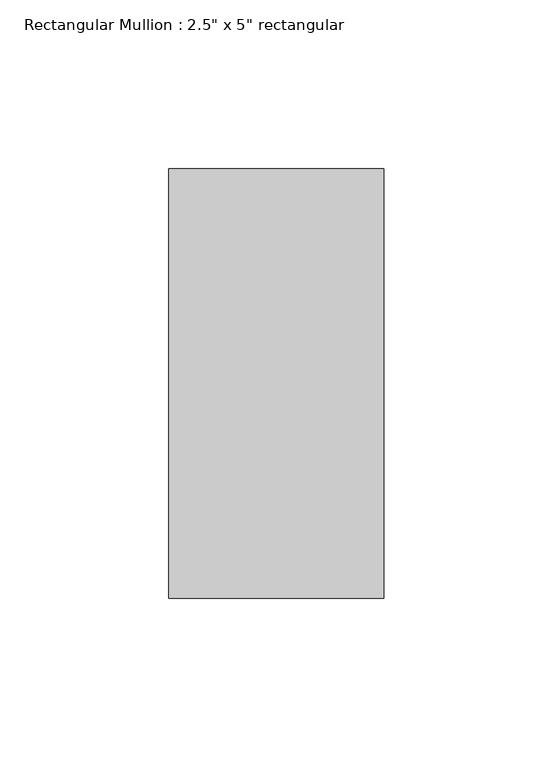
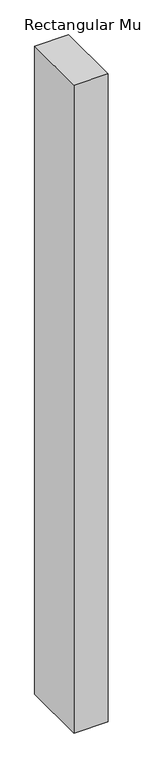
"""IFC4 building model written with IfcOpenShell, lengths in millimetres: member geometry."""

from ifc_helpers import new_model, si_unit, frame, origin, place, context, project, spatial, polyline, outline, extrude, source, transform, mapped, element, save


def member_2b3f0a2a(model_context):
    return source(origin(), model_context, "Body", "SweptSolid", [
        extrude(outline(polyline([(31.75, 63.5), (31.75, -63.5), (-31.75, -63.5), (-31.75, 63.5), (31.75, 63.5)])), frame((0.0, 0.0, -1276.3500001), z_axis=(0.0, 0.0, 1.0), x_axis=(1.0, 0.0, 0.0)), (0.0, 0.0, 1.0), 1276.3500001),
    ])


if __name__ == "__main__":
    model = new_model("IFC4")
    model_context = context("Model", 3, world=origin())
    ifc_project = project(units=[si_unit("LENGTHUNIT", "METRE", prefix="MILLI")], contexts=[model_context])
    site = spatial("IfcSite", under=ifc_project)
    building = spatial("IfcBuilding", under=site)
    placement = place(None, origin())
    member_shape = member_2b3f0a2a(model_context)
    element("IfcMember", 1, ObjectType="Rectangular Mullion : 2.5\" x 5\" rectangular", at=placement, inside=building, context=model_context, shape_type="MappedRepresentation", body=[
        mapped(member_shape, transform((0.0, 0.0, 0.0), x_axis=(1.0, 0.0, 0.0), y_axis=(0.0, 1.0, 0.0), z_axis=(0.0, 0.0, 1.0))),
    ])
    save(model, "model.ifc")

# Revit data of these elements
# Type "Rectangular Mullion : 2.5\" x 5\" rectangular"
#   built-in parameter 1007304 = 0.416667 (stored number, unit not read)
#   built-in parameter 1007301 = 0.104167 (stored number, unit not read)
#   built-in parameter 1007300 = 0.104167 (stored number, unit not read)
# Element 1 (IfcMember, "Rectangular Mullion : 2.5\" x 5\" rectangular")
#   Materials on its faces: "Aluminum"
# Materials
#   "Aluminum": class "Metal", colour RGB 247 247 247, transparency 0, Description = "Aluminum 6061", Cost = 0
